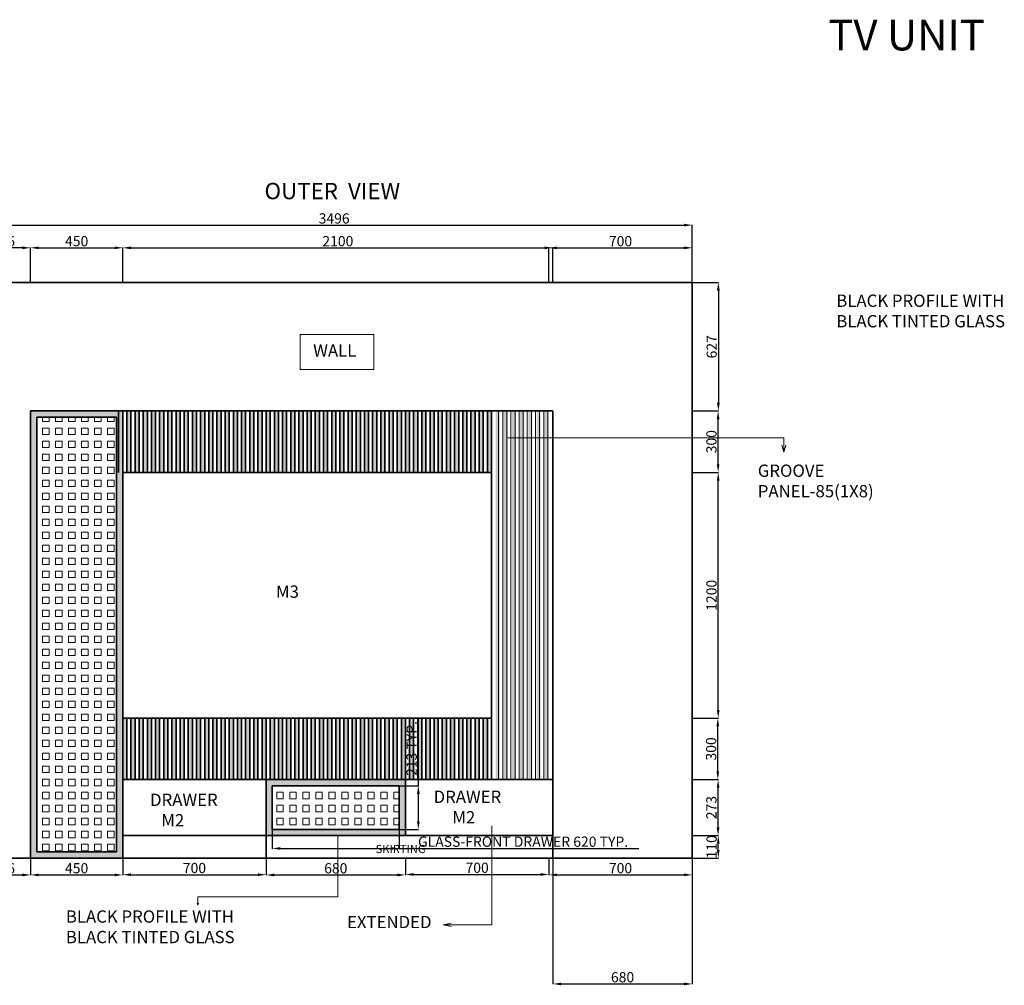
# Model space of a CAD drawing. Units: millimetres. Extents: x 11439 to 24661, y -4767 to -6.
# Tile 2 of 5: x 13922 to 18729, y -4721 to -6. Entities that reach past the tile are written whole.
import ezdxf

# ---------------------------------------------------------------- set-up
doc = ezdxf.new("R2010")
doc.units = ezdxf.units.MM
for name, color, linetype, lineweight in [('A-ANNO-DIMS', 2, 'Continuous', 18), ('A-ANNO-TEXT', 3, 'Continuous', 18), ('A-FURN', 7, 'Continuous', 35), ('A-FURN-PATT', 8, 'Continuous', 13)]:
    doc.layers.add(name, color=color, linetype=linetype, lineweight=lineweight)
doc.styles.get("Standard").update_dxf_attribs({"font": 'arial.ttf'})
doc.dimstyles.new('ISO-25', dxfattribs={"dimtxt": 50, "dimasz": 40, "dimexe": 1.25, "dimexo": 0.625, "dimtad": 1, "dimtxsty": 'Standard', "dimcen": 2.5, "dimadec": 0, "dimazin": 0, "dimtfac": 1, "dimtmove": 0, "dimatfit": 3, "dimfxl": 1, "dimarcsym": 0})

# ---------------------------------------------------------------- blocks, each defined once
blk = doc.blocks.new('*D1')
at = {"layer": 'A-ANNO-DIMS', "color": 0, "lineweight": -2, "transparency": 16777216}
for p, q in [((13708.9, -4100.6), (13708.9, -4183.6)), ((13974.9, -4100.6), (13974.9, -4183.6)), ((13748.9, -4182.3), (13934.9, -4182.3))]:
    blk.add_line(p, q, dxfattribs=at)
at = {"layer": 'A-ANNO-DIMS', "color": 0, "transparency": 16777216}
for points in [[(13748.9, -4175.7), (13748.9, -4189), (13708.9, -4182.3)], [(13934.9, -4175.7), (13934.9, -4189), (13974.9, -4182.3)]]:
    blk.add_solid(points, dxfattribs=at)
at = {"layer": 'Defpoints', "color": 0, "transparency": 16777216}
for p in [(13708.9, -4100), (13974.9, -4100), (13974.9, -4182.3)]:
    blk.add_point(p, dxfattribs=at)
at = {"layer": 'A-ANNO-DIMS', "color": 0, "transparency": 16777216, "insert": (13841.9, -4156.2), "char_height": 50, "attachment_point": 5}
blk.add_mtext('266', dxfattribs=at)
blk = doc.blocks.new('*D2')
at = {"layer": 'A-ANNO-DIMS', "color": 0, "lineweight": -2, "transparency": 16777216}
for p, q in [((13974.9, -4100.6), (13974.9, -4183.6)), ((14424.9, -4100.6), (14424.9, -4183.6)), ((14014.9, -4182.3), (14384.9, -4182.3))]:
    blk.add_line(p, q, dxfattribs=at)
at = {"layer": 'A-ANNO-DIMS', "color": 0, "transparency": 16777216}
for points in [[(14014.9, -4175.7), (14014.9, -4189), (13974.9, -4182.3)], [(14384.9, -4175.7), (14384.9, -4189), (14424.9, -4182.3)]]:
    blk.add_solid(points, dxfattribs=at)
at = {"layer": 'Defpoints', "color": 0, "transparency": 16777216}
for p in [(13974.9, -4100), (14424.9, -4100), (14424.9, -4182.3)]:
    blk.add_point(p, dxfattribs=at)
at = {"layer": 'A-ANNO-DIMS', "color": 0, "transparency": 16777216, "insert": (14199.9, -4156.2), "char_height": 50, "attachment_point": 5}
blk.add_mtext('450', dxfattribs=at)
blk = doc.blocks.new('*D3')
at = {"layer": 'A-ANNO-DIMS', "color": 0, "lineweight": -2, "transparency": 16777216}
for p, q in [((14424.9, -4100.6), (14424.9, -4182.4)), ((15124.9, -4100.6), (15124.9, -4182.4)), ((14464.9, -4181.2), (15084.9, -4181.2))]:
    blk.add_line(p, q, dxfattribs=at)
at = {"layer": 'A-ANNO-DIMS', "color": 0, "transparency": 16777216}
for points in [[(14464.9, -4174.5), (14464.9, -4187.8), (14424.9, -4181.2)], [(15084.9, -4174.5), (15084.9, -4187.8), (15124.9, -4181.2)]]:
    blk.add_solid(points, dxfattribs=at)
at = {"layer": 'Defpoints', "color": 0, "transparency": 16777216}
for p in [(14424.9, -4100), (15124.9, -4100), (15124.9, -4181.2)]:
    blk.add_point(p, dxfattribs=at)
at = {"layer": 'A-ANNO-DIMS', "color": 0, "transparency": 16777216, "insert": (14774.9, -4155), "char_height": 50, "attachment_point": 5}
blk.add_mtext('700', dxfattribs=at)
blk = doc.blocks.new('*D4')
at = {"layer": 'A-ANNO-DIMS', "color": 0, "lineweight": -2, "transparency": 16777216}
for p, q in [((15124.9, -4100.6), (15124.9, -4183.7)), ((15804.9, -4100.6), (15804.9, -4183.7)), ((15164.9, -4182.4), (15764.9, -4182.4))]:
    blk.add_line(p, q, dxfattribs=at)
at = {"layer": 'A-ANNO-DIMS', "color": 0, "transparency": 16777216}
for points in [[(15164.9, -4175.8), (15164.9, -4189.1), (15124.9, -4182.4)], [(15764.9, -4175.8), (15764.9, -4189.1), (15804.9, -4182.4)]]:
    blk.add_solid(points, dxfattribs=at)
at = {"layer": 'Defpoints', "color": 0, "transparency": 16777216}
for p in [(15124.9, -4100), (15804.9, -4100), (15804.9, -4182.4)]:
    blk.add_point(p, dxfattribs=at)
at = {"layer": 'A-ANNO-DIMS', "color": 0, "transparency": 16777216, "insert": (15464.9, -4156.3), "char_height": 50, "attachment_point": 5}
blk.add_mtext('680', dxfattribs=at)
blk = doc.blocks.new('*D5')
at = {"layer": 'A-ANNO-DIMS', "color": 0, "lineweight": -2, "transparency": 16777216}
for p, q in [((15804.9, -4100.6), (15804.9, -4181.3)), ((16504.9, -4100.6), (16504.9, -4181.3)), ((15844.9, -4180), (16464.9, -4180))]:
    blk.add_line(p, q, dxfattribs=at)
at = {"layer": 'A-ANNO-DIMS', "color": 0, "transparency": 16777216}
for points in [[(15844.9, -4173.3), (15844.9, -4186.7), (15804.9, -4180)], [(16464.9, -4173.3), (16464.9, -4186.7), (16504.9, -4180)]]:
    blk.add_solid(points, dxfattribs=at)
at = {"layer": 'Defpoints', "color": 0, "transparency": 16777216}
for p in [(15804.9, -4100), (16504.9, -4100), (16504.9, -4180)]:
    blk.add_point(p, dxfattribs=at)
at = {"layer": 'A-ANNO-DIMS', "color": 0, "transparency": 16777216, "insert": (16154.9, -4153.8), "char_height": 50, "attachment_point": 5}
blk.add_mtext('700', dxfattribs=at)
blk = doc.blocks.new('*D6')
at = {"layer": 'A-ANNO-DIMS', "color": 0, "lineweight": -2, "transparency": 16777216}
for p, q in [((16504.9, -4100.6), (16504.9, -4183.1)), ((17204.9, -4100.6), (17204.9, -4183.1)), ((16544.9, -4181.9), (17164.9, -4181.9))]:
    blk.add_line(p, q, dxfattribs=at)
at = {"layer": 'A-ANNO-DIMS', "color": 0, "transparency": 16777216}
for points in [[(16544.9, -4175.2), (16544.9, -4188.6), (16504.9, -4181.9)], [(17164.9, -4175.2), (17164.9, -4188.6), (17204.9, -4181.9)]]:
    blk.add_solid(points, dxfattribs=at)
at = {"layer": 'Defpoints', "color": 0, "transparency": 16777216}
for p in [(16504.9, -4100), (17204.9, -4100), (17204.9, -4181.9)]:
    blk.add_point(p, dxfattribs=at)
at = {"layer": 'A-ANNO-DIMS', "color": 0, "transparency": 16777216, "insert": (16854.9, -4155.7), "char_height": 50, "attachment_point": 5}
blk.add_mtext('700', dxfattribs=at)
blk = doc.blocks.new('*D7')
at = {"layer": 'A-ANNO-DIMS', "color": 0, "lineweight": -2, "transparency": 16777216}
for p, q in [((17205.5, -3990), (17333.4, -3990)), ((17332.1, -4060), (17332.1, -4030)), ((17205.5, -4100), (17333.4, -4100))]:
    blk.add_line(p, q, dxfattribs=at)
at = {"layer": 'A-ANNO-DIMS', "color": 0, "transparency": 16777216}
for points in [[(17325.5, -4030), (17338.8, -4030), (17332.1, -3990)], [(17325.5, -4060), (17338.8, -4060), (17332.1, -4100)]]:
    blk.add_solid(points, dxfattribs=at)
at = {"layer": 'Defpoints', "color": 0, "transparency": 16777216}
for p in [(17204.9, -3990), (17332.1, -3990), (17204.9, -4100)]:
    blk.add_point(p, dxfattribs=at)
at = {"layer": 'A-ANNO-DIMS', "color": 0, "transparency": 16777216, "insert": (17306, -4045), "char_height": 50, "attachment_point": 5, "rotation": 90}
blk.add_mtext('110', dxfattribs=at)
blk = doc.blocks.new('*D8')
at = {"layer": 'A-ANNO-DIMS', "color": 0, "lineweight": -2, "transparency": 16777216}
for p, q in [((17205.5, -3717), (17332.5, -3717)), ((17331.3, -3950), (17331.3, -3757)), ((17205.5, -3990), (17332.5, -3990))]:
    blk.add_line(p, q, dxfattribs=at)
at = {"layer": 'A-ANNO-DIMS', "color": 0, "transparency": 16777216}
for points in [[(17324.6, -3757), (17338, -3757), (17331.3, -3717)], [(17324.6, -3950), (17338, -3950), (17331.3, -3990)]]:
    blk.add_solid(points, dxfattribs=at)
at = {"layer": 'Defpoints', "color": 0, "transparency": 16777216}
for p in [(17204.9, -3717), (17331.3, -3717), (17204.9, -3990)]:
    blk.add_point(p, dxfattribs=at)
at = {"layer": 'A-ANNO-DIMS', "color": 0, "transparency": 16777216, "insert": (17305.1, -3853.5), "char_height": 50, "attachment_point": 5, "rotation": 90}
blk.add_mtext('273', dxfattribs=at)
blk = doc.blocks.new('*D9')
at = {"layer": 'A-ANNO-DIMS', "color": 0, "lineweight": -2, "transparency": 16777216}
for p, q in [((17205.5, -3417), (17331.1, -3417)), ((17329.9, -3677), (17329.9, -3457)), ((17205.5, -3717), (17331.1, -3717))]:
    blk.add_line(p, q, dxfattribs=at)
at = {"layer": 'A-ANNO-DIMS', "color": 0, "transparency": 16777216}
for points in [[(17323.2, -3457), (17336.5, -3457), (17329.9, -3417)], [(17323.2, -3677), (17336.5, -3677), (17329.9, -3717)]]:
    blk.add_solid(points, dxfattribs=at)
at = {"layer": 'Defpoints', "color": 0, "transparency": 16777216}
for p in [(17204.9, -3417), (17329.9, -3417), (17204.9, -3717)]:
    blk.add_point(p, dxfattribs=at)
at = {"layer": 'A-ANNO-DIMS', "color": 0, "transparency": 16777216, "insert": (17303.7, -3567), "char_height": 50, "attachment_point": 5, "rotation": 90}
blk.add_mtext('300', dxfattribs=at)
blk = doc.blocks.new('*D10')
at = {"layer": 'A-ANNO-DIMS', "color": 0, "lineweight": -2, "transparency": 16777216}
for p, q in [((17205.5, -2217), (17333, -2217)), ((17331.8, -3377), (17331.8, -2257)), ((17205.5, -3417), (17333, -3417))]:
    blk.add_line(p, q, dxfattribs=at)
at = {"layer": 'A-ANNO-DIMS', "color": 0, "transparency": 16777216}
for points in [[(17325.1, -2257), (17338.4, -2257), (17331.8, -2217)], [(17325.1, -3377), (17338.4, -3377), (17331.8, -3417)]]:
    blk.add_solid(points, dxfattribs=at)
at = {"layer": 'Defpoints', "color": 0, "transparency": 16777216}
for p in [(17204.9, -2217), (17331.8, -2217), (17204.9, -3417)]:
    blk.add_point(p, dxfattribs=at)
at = {"layer": 'A-ANNO-DIMS', "color": 0, "transparency": 16777216, "insert": (17305.6, -2817), "char_height": 50, "attachment_point": 5, "rotation": 90}
blk.add_mtext('1200', dxfattribs=at)
blk = doc.blocks.new('*D11')
at = {"layer": 'A-ANNO-DIMS', "color": 0, "lineweight": -2, "transparency": 16777216}
for p, q in [((17209.3, -1917), (17332.6, -1917)), ((17331.4, -2177), (17331.4, -1957)), ((17205.5, -2217), (17332.6, -2217))]:
    blk.add_line(p, q, dxfattribs=at)
at = {"layer": 'A-ANNO-DIMS', "color": 0, "transparency": 16777216}
for points in [[(17324.7, -1957), (17338, -1957), (17331.4, -1917)], [(17324.7, -2177), (17338, -2177), (17331.4, -2217)]]:
    blk.add_solid(points, dxfattribs=at)
at = {"layer": 'Defpoints', "color": 0, "transparency": 16777216}
for p in [(17208.7, -1917), (17331.4, -1917), (17204.9, -2217)]:
    blk.add_point(p, dxfattribs=at)
at = {"layer": 'A-ANNO-DIMS', "color": 0, "transparency": 16777216, "insert": (17305.2, -2067), "char_height": 50, "attachment_point": 5, "rotation": 90}
blk.add_mtext('300', dxfattribs=at)
blk = doc.blocks.new('*D12')
at = {"layer": 'A-ANNO-DIMS', "color": 0, "lineweight": -2, "transparency": 16777216}
for p, q in [((13708.9, -1289.4), (13708.9, -1119.1)), ((13934.9, -1120.3), (13748.9, -1120.3)), ((13974.9, -1289.4), (13974.9, -1119.1))]:
    blk.add_line(p, q, dxfattribs=at)
at = {"layer": 'A-ANNO-DIMS', "color": 0, "transparency": 16777216}
for points in [[(13748.9, -1113.7), (13748.9, -1127), (13708.9, -1120.3)], [(13934.9, -1113.7), (13934.9, -1127), (13974.9, -1120.3)]]:
    blk.add_solid(points, dxfattribs=at)
at = {"layer": 'Defpoints', "color": 0, "transparency": 16777216}
for p in [(13708.9, -1120.3), (13708.9, -1290), (13974.9, -1290)]:
    blk.add_point(p, dxfattribs=at)
at = {"layer": 'A-ANNO-DIMS', "color": 0, "transparency": 16777216, "insert": (13841.9, -1094.2), "char_height": 50, "attachment_point": 5}
blk.add_mtext('266', dxfattribs=at)
blk = doc.blocks.new('*D13')
at = {"layer": 'A-ANNO-DIMS', "color": 0, "lineweight": -2, "transparency": 16777216}
for p, q in [((13974.9, -1289.4), (13974.9, -1119.1)), ((14014.9, -1120.3), (14384.9, -1120.3)), ((14424.9, -1289.4), (14424.9, -1119.1))]:
    blk.add_line(p, q, dxfattribs=at)
at = {"layer": 'A-ANNO-DIMS', "color": 0, "transparency": 16777216}
for points in [[(14014.9, -1113.7), (14014.9, -1127), (13974.9, -1120.3)], [(14384.9, -1113.7), (14384.9, -1127), (14424.9, -1120.3)]]:
    blk.add_solid(points, dxfattribs=at)
at = {"layer": 'Defpoints', "color": 0, "transparency": 16777216}
for p in [(14424.9, -1120.3), (13974.9, -1290), (14424.9, -1290)]:
    blk.add_point(p, dxfattribs=at)
at = {"layer": 'A-ANNO-DIMS', "color": 0, "transparency": 16777216, "insert": (14199.9, -1094.2), "char_height": 50, "attachment_point": 5}
blk.add_mtext('450', dxfattribs=at)
blk = doc.blocks.new('*D14')
at = {"layer": 'A-ANNO-DIMS', "color": 0, "lineweight": -2, "transparency": 16777216}
for p, q in [((14424.9, -1289.4), (14424.9, -1119.2)), ((14464.9, -1120.4), (16484.9, -1120.4)), ((16524.9, -1289.4), (16524.9, -1119.2))]:
    blk.add_line(p, q, dxfattribs=at)
at = {"layer": 'A-ANNO-DIMS', "color": 0, "transparency": 16777216}
for points in [[(14464.9, -1113.8), (14464.9, -1127.1), (14424.9, -1120.4)], [(16484.9, -1113.8), (16484.9, -1127.1), (16524.9, -1120.4)]]:
    blk.add_solid(points, dxfattribs=at)
at = {"layer": 'Defpoints', "color": 0, "transparency": 16777216}
for p in [(16524.9, -1120.4), (14424.9, -1290), (16524.9, -1290)]:
    blk.add_point(p, dxfattribs=at)
at = {"layer": 'A-ANNO-DIMS', "color": 0, "transparency": 16777216, "insert": (15474.9, -1094.3), "char_height": 50, "attachment_point": 5}
blk.add_mtext('2100', dxfattribs=at)
blk = doc.blocks.new('*D15')
at = {"layer": 'A-ANNO-DIMS', "color": 0, "lineweight": -2, "transparency": 16777216}
for p, q in [((16504.9, -1289.4), (16504.9, -1119.2)), ((16544.9, -1120.4), (17164.9, -1120.4)), ((17204.9, -1289.4), (17204.9, -1119.2))]:
    blk.add_line(p, q, dxfattribs=at)
at = {"layer": 'A-ANNO-DIMS', "color": 0, "transparency": 16777216}
for points in [[(16544.9, -1113.8), (16544.9, -1127.1), (16504.9, -1120.4)], [(17164.9, -1113.8), (17164.9, -1127.1), (17204.9, -1120.4)]]:
    blk.add_solid(points, dxfattribs=at)
at = {"layer": 'Defpoints', "color": 0, "transparency": 16777216}
for p in [(17204.9, -1120.4), (16504.9, -1290), (17204.9, -1290)]:
    blk.add_point(p, dxfattribs=at)
at = {"layer": 'A-ANNO-DIMS', "color": 0, "transparency": 16777216, "insert": (16854.9, -1094.3), "char_height": 50, "attachment_point": 5}
blk.add_mtext('700', dxfattribs=at)
blk = doc.blocks.new('*D16')
at = {"layer": 'A-ANNO-DIMS', "color": 0, "lineweight": -2, "transparency": 16777216}
for p, q in [((17205.5, -1290), (17333.9, -1290)), ((17332.6, -1330), (17332.6, -1877)), ((17209.3, -1917), (17333.9, -1917))]:
    blk.add_line(p, q, dxfattribs=at)
at = {"layer": 'A-ANNO-DIMS', "color": 0, "transparency": 16777216}
for points in [[(17325.9, -1330), (17339.3, -1330), (17332.6, -1290)], [(17325.9, -1877), (17339.3, -1877), (17332.6, -1917)]]:
    blk.add_solid(points, dxfattribs=at)
at = {"layer": 'Defpoints', "color": 0, "transparency": 16777216}
for p in [(17204.9, -1290), (17208.7, -1917), (17332.6, -1917)]:
    blk.add_point(p, dxfattribs=at)
at = {"layer": 'A-ANNO-DIMS', "color": 0, "transparency": 16777216, "insert": (17306.5, -1603.5), "char_height": 50, "attachment_point": 5, "rotation": 90}
blk.add_mtext('627', dxfattribs=at)
blk = doc.blocks.new('DRAWER-GLASS-FRONT')
for p, q in [((0, 213), (620, 213)), ((0, 0), (0, 213)), ((620, 0), (620, 213)), ((0, 0), (620, 0))]:
    blk.add_line(p, q)
blk = doc.blocks.new('*D49')
at = {"layer": 'A-ANNO-DIMS', "color": 0, "lineweight": -2, "transparency": 16777216}
for p, q in [((15154.9, -3960.6), (15154.9, -4054.2)), ((15774.9, -3960.6), (15774.9, -4054.2)), ((15194.9, -4053), (15734.9, -4053)), ((15774.9, -4053), (16943.6, -4053))]:
    blk.add_line(p, q, dxfattribs=at)
at = {"layer": 'A-ANNO-DIMS', "color": 0, "transparency": 16777216}
for points in [[(15194.9, -4046.3), (15194.9, -4059.7), (15154.9, -4053)], [(15734.9, -4046.3), (15734.9, -4059.7), (15774.9, -4053)]]:
    blk.add_solid(points, dxfattribs=at)
at = {"layer": 'Defpoints', "color": 0, "transparency": 16777216}
for p in [(15154.9, -3960), (15774.9, -3960), (15774.9, -4053)]:
    blk.add_point(p, dxfattribs=at)
at = {"layer": 'A-ANNO-DIMS', "color": 0, "transparency": 16777216, "insert": (16379.3, -4026.5), "char_height": 50, "attachment_point": 5}
blk.add_mtext('GLASS-FRONT DRAWER 620 TYP.', dxfattribs=at)
blk = doc.blocks.new('*D50')
at = {"layer": 'A-ANNO-DIMS', "color": 0, "lineweight": -2, "transparency": 16777216}
for p, q in [((15867.9, -3747), (15867.9, -3422.7)), ((15775.5, -3747), (15869.2, -3747)), ((15867.9, -3920), (15867.9, -3787)), ((15775.5, -3960), (15869.2, -3960))]:
    blk.add_line(p, q, dxfattribs=at)
at = {"layer": 'A-ANNO-DIMS', "color": 0, "transparency": 16777216}
for points in [[(15861.2, -3787), (15874.6, -3787), (15867.9, -3747)], [(15861.2, -3920), (15874.6, -3920), (15867.9, -3960)]]:
    blk.add_solid(points, dxfattribs=at)
at = {"layer": 'Defpoints', "color": 0, "transparency": 16777216}
for p in [(15774.9, -3747), (15867.9, -3747), (15774.9, -3960)]:
    blk.add_point(p, dxfattribs=at)
at = {"layer": 'A-ANNO-DIMS', "color": 0, "transparency": 16777216, "insert": (15841.7, -3564.8), "char_height": 50, "attachment_point": 5, "rotation": 90}
blk.add_mtext('213 TYP.', dxfattribs=at)
blk = doc.blocks.new('*D57')
at = {"layer": 'A-ANNO-DIMS', "color": 0, "lineweight": -2, "transparency": 16777216}
for p, q in [((16524.9, -4100.6), (16524.9, -4715.8)), ((17204.9, -4100.6), (17204.9, -4715.8)), ((16564.9, -4714.6), (17164.9, -4714.6))]:
    blk.add_line(p, q, dxfattribs=at)
at = {"layer": 'A-ANNO-DIMS', "color": 0, "transparency": 16777216}
for points in [[(16564.9, -4707.9), (16564.9, -4721.2), (16524.9, -4714.6)], [(17164.9, -4707.9), (17164.9, -4721.2), (17204.9, -4714.6)]]:
    blk.add_solid(points, dxfattribs=at)
at = {"layer": 'Defpoints', "color": 0, "transparency": 16777216}
for p in [(16524.9, -4100), (17204.9, -4100), (17204.9, -4714.6)]:
    blk.add_point(p, dxfattribs=at)
at = {"layer": 'A-ANNO-DIMS', "color": 0, "transparency": 16777216, "insert": (16864.9, -4688.4), "char_height": 50, "attachment_point": 5}
blk.add_mtext('680', dxfattribs=at)
blk = doc.blocks.new('*D58')
at = {"layer": 'A-ANNO-DIMS', "color": 0, "lineweight": -2, "transparency": 16777216}
for p, q in [((13708.9, -1289.4), (13708.9, -1008.2)), ((17204.9, -1289.4), (17204.9, -1008.2)), ((13748.9, -1009.5), (17164.9, -1009.5))]:
    blk.add_line(p, q, dxfattribs=at)
at = {"layer": 'A-ANNO-DIMS', "color": 0, "transparency": 16777216}
for points in [[(13748.9, -1002.8), (13748.9, -1016.2), (13708.9, -1009.5)], [(17164.9, -1002.8), (17164.9, -1016.2), (17204.9, -1009.5)]]:
    blk.add_solid(points, dxfattribs=at)
at = {"layer": 'Defpoints', "color": 0, "transparency": 16777216}
for p in [(17204.9, -1009.5), (13708.9, -1290), (17204.9, -1290)]:
    blk.add_point(p, dxfattribs=at)
at = {"layer": 'A-ANNO-DIMS', "color": 0, "transparency": 16777216, "insert": (15456.9, -983.3), "char_height": 50, "attachment_point": 5}
blk.add_mtext('3496', dxfattribs=at)

msp = doc.modelspace()

# ---------------------------------------------------------------- hatches: boundary and pattern name
at = {"layer": 'A-FURN-PATT'}
h = msp.add_hatch(color=256, dxfattribs=at)
h.dxf.hatch_style = 1
h.paths.add_polyline_path([(13974.915, -4099.995), (14424.915, -4099.995), (14424.915, -1916.995), (13974.915, -1916.995)])
h.paths.add_polyline_path([(14004.915, -1946.995), (14394.915, -1946.995), (14394.915, -4069.995), (14004.915, -4069.995)], flags=16)
h = msp.add_hatch(color=256, dxfattribs=at)
h.dxf.hatch_style = 1
h.paths.add_polyline_path([(14464.915, -1916.995), (14444.915, -1916.995), (14444.915, -2216.995), (14464.915, -2216.995)])
h = msp.add_hatch(color=256, dxfattribs=at)
h.dxf.hatch_style = 1
h.paths.add_polyline_path([(14504.915, -1916.995), (14484.915, -1916.995), (14484.915, -2216.995), (14504.915, -2216.995)])
h.paths.add_polyline_path([(14544.915, -1916.995), (14524.915, -1916.995), (14524.915, -2216.995), (14544.915, -2216.995)])
h.paths.add_polyline_path([(14584.915, -1916.995), (14564.915, -1916.995), (14564.915, -2216.995), (14584.915, -2216.995)])
h.paths.add_polyline_path([(14624.915, -1916.995), (14604.915, -1916.995), (14604.915, -2216.995), (14624.915, -2216.995)])
h.paths.add_polyline_path([(14664.915, -1916.995), (14644.915, -1916.995), (14644.915, -2216.995), (14664.915, -2216.995)])
h.paths.add_polyline_path([(14704.915, -1916.995), (14684.915, -1916.995), (14684.915, -2216.995), (14704.915, -2216.995)])
h.paths.add_polyline_path([(14744.915, -1916.995), (14724.915, -1916.995), (14724.915, -2216.995), (14744.915, -2216.995)])
h.paths.add_polyline_path([(14784.915, -1916.995), (14764.915, -1916.995), (14764.915, -2216.995), (14784.915, -2216.995)])
h.paths.add_polyline_path([(14824.915, -1916.995), (14804.915, -1916.995), (14804.915, -2216.995), (14824.915, -2216.995)])
h.paths.add_polyline_path([(14864.915, -1916.995), (14844.915, -1916.995), (14844.915, -2216.995), (14864.915, -2216.995)])
h.paths.add_polyline_path([(14904.915, -1916.995), (14884.915, -1916.995), (14884.915, -2216.995), (14904.915, -2216.995)])
h.paths.add_polyline_path([(14944.915, -1916.995), (14924.915, -1916.995), (14924.915, -2216.995), (14944.915, -2216.995)])
h.paths.add_polyline_path([(14984.915, -1916.995), (14964.915, -1916.995), (14964.915, -2216.995), (14984.915, -2216.995)])
h.paths.add_polyline_path([(15024.915, -1916.995), (15004.915, -1916.995), (15004.915, -2216.995), (15024.915, -2216.995)])
h.paths.add_polyline_path([(15064.915, -1916.995), (15044.915, -1916.995), (15044.915, -2216.995), (15064.915, -2216.995)])
h.paths.add_polyline_path([(15104.915, -1916.995), (15084.915, -1916.995), (15084.915, -2216.995), (15104.915, -2216.995)])
h.paths.add_polyline_path([(15144.915, -1916.995), (15124.915, -1916.995), (15124.915, -2216.995), (15144.915, -2216.995)])
h.paths.add_polyline_path([(15184.915, -1916.995), (15164.915, -1916.995), (15164.915, -2216.995), (15184.915, -2216.995)])
h.paths.add_polyline_path([(15224.915, -1916.995), (15204.915, -1916.995), (15204.915, -2216.995), (15224.915, -2216.995)])
h.paths.add_polyline_path([(15264.915, -1916.995), (15244.915, -1916.995), (15244.915, -2216.995), (15264.915, -2216.995)])
h.paths.add_polyline_path([(15304.915, -1916.995), (15284.915, -1916.995), (15284.915, -2216.995), (15304.915, -2216.995)])
h.paths.add_polyline_path([(15344.915, -1916.995), (15324.915, -1916.995), (15324.915, -2216.995), (15344.915, -2216.995)])
h.paths.add_polyline_path([(15384.915, -1916.995), (15364.915, -1916.995), (15364.915, -2216.995), (15384.915, -2216.995)])
h.paths.add_polyline_path([(15424.915, -1916.995), (15404.915, -1916.995), (15404.915, -2216.995), (15424.915, -2216.995)])
h.paths.add_polyline_path([(15464.915, -1916.995), (15444.915, -1916.995), (15444.915, -2216.995), (15464.915, -2216.995)])
h.paths.add_polyline_path([(15504.915, -1916.995), (15484.915, -1916.995), (15484.915, -2216.995), (15504.915, -2216.995)])
h.paths.add_polyline_path([(15544.915, -1916.995), (15524.915, -1916.995), (15524.915, -2216.995), (15544.915, -2216.995)])
h.paths.add_polyline_path([(15584.915, -1916.995), (15564.915, -1916.995), (15564.915, -2216.995), (15584.915, -2216.995)])
h.paths.add_polyline_path([(15624.915, -1916.995), (15604.915, -1916.995), (15604.915, -2216.995), (15624.915, -2216.995)])
h.paths.add_polyline_path([(15664.915, -1916.995), (15644.915, -1916.995), (15644.915, -2216.995), (15664.915, -2216.995)])
h.paths.add_polyline_path([(15704.915, -1916.995), (15684.915, -1916.995), (15684.915, -2216.995), (15704.915, -2216.995)])
h.paths.add_polyline_path([(15744.915, -1916.995), (15724.915, -1916.995), (15724.915, -2216.995), (15744.915, -2216.995)])
h.paths.add_polyline_path([(15784.915, -1916.995), (15764.915, -1916.995), (15764.915, -2216.995), (15784.915, -2216.995)])
h.paths.add_polyline_path([(15824.915, -1916.995), (15804.915, -1916.995), (15804.915, -2216.995), (15824.915, -2216.995)])
h.paths.add_polyline_path([(15864.915, -1916.995), (15844.915, -1916.995), (15844.915, -2216.995), (15864.915, -2216.995)])
h.paths.add_polyline_path([(15904.915, -1916.995), (15884.915, -1916.995), (15884.915, -2216.995), (15904.915, -2216.995)])
h.paths.add_polyline_path([(15944.915, -1916.995), (15924.915, -1916.995), (15924.915, -2216.995), (15944.915, -2216.995)])
h.paths.add_polyline_path([(15984.915, -1916.995), (15964.915, -1916.995), (15964.915, -2216.995), (15984.915, -2216.995)])
h.paths.add_polyline_path([(16024.915, -1916.995), (16004.915, -1916.995), (16004.915, -2216.995), (16024.915, -2216.995)])
h.paths.add_polyline_path([(16064.915, -1916.995), (16044.915, -1916.995), (16044.915, -2216.995), (16064.915, -2216.995)])
h.paths.add_polyline_path([(16104.915, -1916.995), (16084.915, -1916.995), (16084.915, -2216.995), (16104.915, -2216.995)])
h.paths.add_polyline_path([(16144.915, -1916.995), (16124.915, -1916.995), (16124.915, -2216.995), (16144.915, -2216.995)])
h.paths.add_polyline_path([(16184.915, -1916.995), (16164.915, -1916.995), (16164.915, -2216.995), (16184.915, -2216.995)])
h.paths.add_polyline_path([(16224.915, -1916.995), (16204.915, -1916.995), (16204.915, -2216.995), (16224.915, -2216.995)])
h = msp.add_hatch(color=256, dxfattribs=at)
h.dxf.hatch_style = 1
h.paths.add_polyline_path([(16264.915, -1916.995), (16244.915, -1916.995), (16244.915, -3716.995), (16264.915, -3716.995)])
h.paths.add_polyline_path([(16304.915, -1916.995), (16284.915, -1916.995), (16284.915, -3716.995), (16304.915, -3716.995)])
h.paths.add_polyline_path([(16344.915, -1916.995), (16324.915, -1916.995), (16324.915, -2047.953), (16344.915, -2047.953)])
h.paths.add_polyline_path([(16344.915, -2047.953), (16324.915, -2047.953), (16324.915, -3716.995), (16344.915, -3716.995)])
h.paths.add_polyline_path([(16384.915, -2047.953), (16364.915, -2047.953), (16364.915, -3716.995), (16384.915, -3716.995)])
h.paths.add_polyline_path([(16384.915, -1916.995), (16364.915, -1916.995), (16364.915, -2047.953), (16384.915, -2047.953)])
h.paths.add_polyline_path([(16424.915, -1916.995), (16404.915, -1916.995), (16404.915, -2047.953), (16424.915, -2047.953)])
h.paths.add_polyline_path([(16424.915, -2047.953), (16404.915, -2047.953), (16404.915, -3716.995), (16424.915, -3716.995)])
h.paths.add_polyline_path([(16464.915, -2047.953), (16444.915, -2047.953), (16444.915, -3716.995), (16464.915, -3716.995)])
h.paths.add_polyline_path([(16464.915, -1916.995), (16444.915, -1916.995), (16444.915, -2047.953), (16464.915, -2047.953)])
h.paths.add_polyline_path([(16504.915, -2047.953), (16484.915, -2047.953), (16484.915, -3716.995), (16504.915, -3716.995)])
h.paths.add_polyline_path([(16504.915, -1916.995), (16484.915, -1916.995), (16484.915, -2047.953), (16504.915, -2047.953)])
h = msp.add_hatch(dxfattribs=at)
h.set_pattern_fill('ANSI31', color=256, scale=6.29921, angle=45, style=0)
h.paths.add_polyline_path([(16244.915, -3716.995), (16504.915, -3716.995), (16504.915, -1916.995), (16244.915, -1916.995)])
h = msp.add_hatch(dxfattribs=at)
h.set_pattern_fill('SQUARE', color=256, scale=10)
h.paths.add_polyline_path([(14394.915, -1946.995), (14004.915, -1946.995), (14004.915, -4069.995), (14394.915, -4069.995)])
h = msp.add_hatch(color=256, dxfattribs=at)
h.dxf.hatch_style = 1
h.paths.add_polyline_path([(14444.915, -3416.995), (14424.915, -3416.995), (14424.915, -3716.995), (14444.915, -3716.995)])
h.paths.add_polyline_path([(14484.915, -3416.995), (14464.915, -3416.995), (14464.915, -3716.995), (14484.915, -3716.995)])
h.paths.add_polyline_path([(14524.915, -3416.995), (14504.915, -3416.995), (14504.915, -3716.995), (14524.915, -3716.995)])
h.paths.add_polyline_path([(14564.915, -3416.995), (14544.915, -3416.995), (14544.915, -3716.995), (14564.915, -3716.995)])
h.paths.add_polyline_path([(14604.915, -3416.995), (14584.915, -3416.995), (14584.915, -3716.995), (14604.915, -3716.995)])
h.paths.add_polyline_path([(14644.915, -3416.995), (14624.915, -3416.995), (14624.915, -3716.995), (14644.915, -3716.995)])
h.paths.add_polyline_path([(14684.915, -3416.995), (14664.915, -3416.995), (14664.915, -3716.995), (14684.915, -3716.995)])
h.paths.add_polyline_path([(14724.915, -3416.995), (14704.915, -3416.995), (14704.915, -3716.995), (14724.915, -3716.995)])
h.paths.add_polyline_path([(14764.915, -3416.995), (14744.915, -3416.995), (14744.915, -3716.995), (14764.915, -3716.995)])
h.paths.add_polyline_path([(14804.915, -3416.995), (14784.915, -3416.995), (14784.915, -3716.995), (14804.915, -3716.995)])
h.paths.add_polyline_path([(14844.915, -3416.995), (14824.915, -3416.995), (14824.915, -3716.995), (14844.915, -3716.995)])
h.paths.add_polyline_path([(14884.915, -3416.995), (14864.915, -3416.995), (14864.915, -3716.995), (14884.915, -3716.995)])
h.paths.add_polyline_path([(14924.915, -3416.995), (14904.915, -3416.995), (14904.915, -3716.995), (14924.915, -3716.995)])
h.paths.add_polyline_path([(14964.915, -3416.995), (14944.915, -3416.995), (14944.915, -3716.995), (14964.915, -3716.995)])
h.paths.add_polyline_path([(15004.915, -3416.995), (14984.915, -3416.995), (14984.915, -3716.995), (15004.915, -3716.995)])
h.paths.add_polyline_path([(15044.915, -3416.995), (15024.915, -3416.995), (15024.915, -3716.995), (15044.915, -3716.995)])
h.paths.add_polyline_path([(15084.915, -3416.995), (15064.915, -3416.995), (15064.915, -3716.995), (15084.915, -3716.995)])
h.paths.add_polyline_path([(15124.915, -3416.995), (15104.915, -3416.995), (15104.915, -3716.995), (15124.915, -3716.995)])
h.paths.add_polyline_path([(15164.915, -3416.995), (15144.915, -3416.995), (15144.915, -3716.995), (15164.915, -3716.995)])
h.paths.add_polyline_path([(15204.915, -3416.995), (15184.915, -3416.995), (15184.915, -3716.995), (15204.915, -3716.995)])
h.paths.add_polyline_path([(15244.915, -3416.995), (15224.915, -3416.995), (15224.915, -3716.995), (15244.915, -3716.995)])
h.paths.add_polyline_path([(15284.915, -3416.995), (15264.915, -3416.995), (15264.915, -3716.995), (15284.915, -3716.995)])
h.paths.add_polyline_path([(15324.915, -3416.995), (15304.915, -3416.995), (15304.915, -3716.995), (15324.915, -3716.995)])
h.paths.add_polyline_path([(15364.915, -3416.995), (15344.915, -3416.995), (15344.915, -3716.995), (15364.915, -3716.995)])
h.paths.add_polyline_path([(15404.915, -3416.995), (15384.915, -3416.995), (15384.915, -3716.995), (15404.915, -3716.995)])
h.paths.add_polyline_path([(15444.915, -3416.995), (15424.915, -3416.995), (15424.915, -3716.995), (15444.915, -3716.995)])
h.paths.add_polyline_path([(15484.915, -3416.995), (15464.915, -3416.995), (15464.915, -3716.995), (15484.915, -3716.995)])
h.paths.add_polyline_path([(15524.915, -3416.995), (15504.915, -3416.995), (15504.915, -3716.995), (15524.915, -3716.995)])
h.paths.add_polyline_path([(15564.915, -3416.995), (15544.915, -3416.995), (15544.915, -3716.995), (15564.915, -3716.995)])
h.paths.add_polyline_path([(15604.915, -3416.995), (15584.915, -3416.995), (15584.915, -3716.995), (15604.915, -3716.995)])
h.paths.add_polyline_path([(15644.915, -3416.995), (15624.915, -3416.995), (15624.915, -3716.995), (15644.915, -3716.995)])
h.paths.add_polyline_path([(15684.915, -3416.995), (15664.915, -3416.995), (15664.915, -3716.995), (15684.915, -3716.995)])
h.paths.add_polyline_path([(15724.915, -3416.995), (15704.915, -3416.995), (15704.915, -3716.995), (15724.915, -3716.995)])
h.paths.add_polyline_path([(15764.915, -3416.995), (15744.915, -3416.995), (15744.915, -3716.995), (15764.915, -3716.995)])
h.paths.add_polyline_path([(15804.915, -3416.995), (15784.915, -3416.995), (15784.915, -3716.995), (15804.915, -3716.995)])
h.paths.add_polyline_path([(15844.915, -3416.995), (15824.915, -3416.995), (15824.915, -3716.995), (15844.915, -3716.995)])
h.paths.add_polyline_path([(15884.915, -3416.995), (15864.915, -3416.995), (15864.915, -3716.995), (15884.915, -3716.995)])
h.paths.add_polyline_path([(15924.915, -3416.995), (15904.915, -3416.995), (15904.915, -3716.995), (15924.915, -3716.995)])
h.paths.add_polyline_path([(15964.915, -3416.995), (15944.915, -3416.995), (15944.915, -3716.995), (15964.915, -3716.995)])
h.paths.add_polyline_path([(16004.915, -3416.995), (15984.915, -3416.995), (15984.915, -3716.995), (16004.915, -3716.995)])
h.paths.add_polyline_path([(16044.915, -3416.995), (16024.915, -3416.995), (16024.915, -3716.995), (16044.915, -3716.995)])
h.paths.add_polyline_path([(16084.915, -3416.995), (16064.915, -3416.995), (16064.915, -3716.995), (16084.915, -3716.995)])
h.paths.add_polyline_path([(16124.915, -3416.995), (16104.915, -3416.995), (16104.915, -3716.995), (16124.915, -3716.995)])
h.paths.add_polyline_path([(16164.915, -3416.995), (16144.915, -3416.995), (16144.915, -3716.995), (16164.915, -3716.995)])
h.paths.add_polyline_path([(16204.915, -3416.995), (16184.915, -3416.995), (16184.915, -3716.995), (16204.915, -3716.995)])
h = msp.add_hatch(color=256, dxfattribs=at)
h.dxf.hatch_style = 1
h.paths.add_polyline_path([(15804.915, -3989.995), (15804.915, -3716.995), (15124.915, -3716.995), (15124.915, -3989.995)])
h.paths.add_polyline_path([(15154.915, -3959.995), (15154.915, -3746.995), (15774.915, -3746.995), (15774.915, -3959.995)], flags=16)
h = msp.add_hatch(dxfattribs=at)
h.set_pattern_fill('SQUARE', color=256, scale=10)
h.paths.add_polyline_path([(15774.915, -3746.995), (15154.915, -3746.995), (15154.915, -3959.995), (15774.915, -3959.995)])

# ---------------------------------------------------------------- linework, layer by layer
at = {"layer": 'A-ANNO-TEXT'}
for p, q in [((16304.915, -2047.953), (16304.915, -2047.953)), ((16304.915, -2047.953), (17651.688, -2047.953)), ((17651.688, -2047.953), (17651.688, -2118.822)), ((17651.688, -2118.822), (17642.208, -2084.333)), ((17651.688, -2118.822), (17661.416, -2083.419)), ((16226.224, -3942.125), (16226.224, -4425.71)), ((15474.915, -3989.995), (15474.915, -4289.242)), ((14792.131, -4329.892), (14788.722, -4319.304)), ((15474.915, -4289.242), (14792.131, -4289.242)), ((14792.131, -4289.242), (14792.131, -4329.892)), ((14792.131, -4329.892), (14795.396, -4319.622)), ((15989.686, -4425.71), (16028.206, -4417.919)), ((16226.224, -4425.71), (15989.686, -4425.71)), ((15989.686, -4425.71), (16029.321, -4434.071))]:
    msp.add_line(p, q, dxfattribs=at)
msp.add_lwpolyline([(15291.366, -1544.351), (15650.752, -1544.351), (15650.752, -1713.672), (15291.366, -1713.672)], close=True, dxfattribs=at)
at = {"layer": 'A-FURN'}
for p, q in [((13708.915, -1289.995), (17204.915, -1289.995)), ((17204.915, -4099.995), (17204.915, -1289.995)), ((13974.915, -4099.995), (13974.915, -1916.995)), ((13974.915, -1916.995), (16524.915, -1916.995)), ((14404.915, -2216.995), (14404.915, -1916.995)), ((14424.915, -4099.995), (14424.915, -1916.995)), ((14424.915, -2216.995), (14424.915, -1916.995)), ((14444.915, -2216.995), (14444.915, -1916.995)), ((14464.915, -2216.995), (14464.915, -1916.995)), ((14484.915, -2216.995), (14484.915, -1916.995)), ((14504.915, -2216.995), (14504.915, -1916.995)), ((14524.915, -2216.995), (14524.915, -1916.995)), ((14544.915, -2216.995), (14544.915, -1916.995)), ((14564.915, -2216.995), (14564.915, -1916.995)), ((14584.915, -2216.995), (14584.915, -1916.995)), ((14604.915, -2216.995), (14604.915, -1916.995)), ((14624.915, -2216.995), (14624.915, -1916.995)), ((14644.915, -2216.995), (14644.915, -1916.995)), ((14664.915, -2216.995), (14664.915, -1916.995)), ((14684.915, -2216.995), (14684.915, -1916.995)), ((14704.915, -2216.995), (14704.915, -1916.995)), ((14724.915, -2216.995), (14724.915, -1916.995)), ((14744.915, -2216.995), (14744.915, -1916.995)), ((14764.915, -2216.995), (14764.915, -1916.995)), ((14784.915, -2216.995), (14784.915, -1916.995)), ((14804.915, -2216.995), (14804.915, -1916.995)), ((14824.915, -2216.995), (14824.915, -1916.995)), ((14844.915, -2216.995), (14844.915, -1916.995)), ((14864.915, -2216.995), (14864.915, -1916.995)), ((14884.915, -2216.995), (14884.915, -1916.995)), ((14904.915, -2216.995), (14904.915, -1916.995)), ((14924.915, -2216.995), (14924.915, -1916.995)), ((14944.915, -2216.995), (14944.915, -1916.995)), ((14964.915, -2216.995), (14964.915, -1916.995)), ((14984.915, -2216.995), (14984.915, -1916.995)), ((15004.915, -2216.995), (15004.915, -1916.995)), ((15024.915, -2216.995), (15024.915, -1916.995)), ((15044.915, -2216.995), (15044.915, -1916.995)), ((15064.915, -2216.995), (15064.915, -1916.995)), ((15084.915, -2216.995), (15084.915, -1916.995)), ((15104.915, -2216.995), (15104.915, -1916.995)), ((15124.915, -2216.995), (15124.915, -1916.995)), ((15144.915, -2216.995), (15144.915, -1916.995)), ((15164.915, -2216.995), (15164.915, -1916.995)), ((15184.915, -2216.995), (15184.915, -1916.995)), ((15204.915, -2216.995), (15204.915, -1916.995)), ((15224.915, -2216.995), (15224.915, -1916.995)), ((15244.915, -2216.995), (15244.915, -1916.995)), ((15264.915, -2216.995), (15264.915, -1916.995)), ((15284.915, -2216.995), (15284.915, -1916.995)), ((15304.915, -2216.995), (15304.915, -1916.995)), ((15324.915, -2216.995), (15324.915, -1916.995)), ((15344.915, -2216.995), (15344.915, -1916.995)), ((15364.915, -2216.995), (15364.915, -1916.995)), ((15384.915, -2216.995), (15384.915, -1916.995)), ((15404.915, -2216.995), (15404.915, -1916.995)), ((15424.915, -2216.995), (15424.915, -1916.995)), ((15444.915, -2216.995), (15444.915, -1916.995)), ((15464.915, -2216.995), (15464.915, -1916.995)), ((15484.915, -2216.995), (15484.915, -1916.995)), ((15504.915, -2216.995), (15504.915, -1916.995)), ((15524.915, -2216.995), (15524.915, -1916.995)), ((15544.915, -2216.995), (15544.915, -1916.995)), ((15564.915, -2216.995), (15564.915, -1916.995)), ((15584.915, -2216.995), (15584.915, -1916.995)), ((15604.915, -2216.995), (15604.915, -1916.995)), ((15624.915, -2216.995), (15624.915, -1916.995)), ((15644.915, -2216.995), (15644.915, -1916.995)), ((15664.915, -2216.995), (15664.915, -1916.995)), ((15684.915, -2216.995), (15684.915, -1916.995)), ((15704.915, -2216.995), (15704.915, -1916.995)), ((15724.915, -2216.995), (15724.915, -1916.995)), ((15744.915, -2216.995), (15744.915, -1916.995)), ((15764.915, -2216.995), (15764.915, -1916.995)), ((15784.915, -2216.995), (15784.915, -1916.995)), ((15804.915, -2216.995), (15804.915, -1916.995)), ((15824.915, -2216.995), (15824.915, -1916.995)), ((15844.915, -2216.995), (15844.915, -1916.995)), ((15864.915, -2216.995), (15864.915, -1916.995)), ((15884.915, -2216.995), (15884.915, -1916.995)), ((15904.915, -2216.995), (15904.915, -1916.995)), ((15924.915, -2216.995), (15924.915, -1916.995)), ((15944.915, -2216.995), (15944.915, -1916.995)), ((15964.915, -2216.995), (15964.915, -1916.995)), ((15984.915, -2216.995), (15984.915, -1916.995)), ((16004.915, -2216.995), (16004.915, -1916.995)), ((16024.915, -2216.995), (16024.915, -1916.995)), ((16044.915, -2216.995), (16044.915, -1916.995)), ((16064.915, -2216.995), (16064.915, -1916.995)), ((16084.915, -2216.995), (16084.915, -1916.995)), ((16104.915, -2216.995), (16104.915, -1916.995)), ((16124.915, -2216.995), (16124.915, -1916.995)), ((16144.915, -2216.995), (16144.915, -1916.995)), ((16164.915, -2216.995), (16164.915, -1916.995)), ((16184.915, -2216.995), (16184.915, -1916.995)), ((16204.915, -2216.995), (16204.915, -1916.995)), ((16224.915, -2216.995), (16224.915, -1916.995)), ((16524.915, -4099.995), (16524.915, -1916.995)), ((14004.915, -4069.995), (14004.915, -1946.995)), ((14004.915, -1946.995), (14394.915, -1946.995)), ((14394.915, -4069.995), (14394.915, -1946.995)), ((14424.915, -2216.995), (16224.915, -2216.995)), ((16224.915, -3416.995), (16224.915, -2216.995)), ((14424.915, -3416.995), (16224.915, -3416.995)), ((14444.915, -3716.995), (14444.915, -3416.995)), ((14464.915, -3716.995), (14464.915, -3416.995)), ((14484.915, -3716.995), (14484.915, -3416.995)), ((14504.915, -3716.995), (14504.915, -3416.995)), ((14524.915, -3716.995), (14524.915, -3416.995)), ((14544.915, -3716.995), (14544.915, -3416.995)), ((14564.915, -3716.995), (14564.915, -3416.995)), ((14584.915, -3716.995), (14584.915, -3416.995)), ((14604.915, -3716.995), (14604.915, -3416.995)), ((14624.915, -3716.995), (14624.915, -3416.995)), ((14644.915, -3716.995), (14644.915, -3416.995)), ((14664.915, -3716.995), (14664.915, -3416.995)), ((14684.915, -3716.995), (14684.915, -3416.995)), ((14704.915, -3716.995), (14704.915, -3416.995)), ((14724.915, -3716.995), (14724.915, -3416.995)), ((14744.915, -3716.995), (14744.915, -3416.995)), ((14764.915, -3716.995), (14764.915, -3416.995)), ((14784.915, -3716.995), (14784.915, -3416.995)), ((14804.915, -3716.995), (14804.915, -3416.995)), ((14824.915, -3716.995), (14824.915, -3416.995)), ((14844.915, -3716.995), (14844.915, -3416.995)), ((14864.915, -3716.995), (14864.915, -3416.995)), ((14884.915, -3716.995), (14884.915, -3416.995)), ((14904.915, -3716.995), (14904.915, -3416.995)), ((14924.915, -3716.995), (14924.915, -3416.995)), ((14944.915, -3716.995), (14944.915, -3416.995)), ((14964.915, -3716.995), (14964.915, -3416.995)), ((14984.915, -3716.995), (14984.915, -3416.995)), ((15004.915, -3716.995), (15004.915, -3416.995)), ((15024.915, -3716.995), (15024.915, -3416.995)), ((15044.915, -3716.995), (15044.915, -3416.995)), ((15064.915, -3716.995), (15064.915, -3416.995)), ((15084.915, -3716.995), (15084.915, -3416.995)), ((15104.915, -3716.995), (15104.915, -3416.995)), ((15124.915, -3716.995), (15124.915, -3416.995)), ((15144.915, -3716.995), (15144.915, -3416.995)), ((15164.915, -3716.995), (15164.915, -3416.995)), ((15184.915, -3716.995), (15184.915, -3416.995)), ((15204.915, -3716.995), (15204.915, -3416.995)), ((15224.915, -3716.995), (15224.915, -3416.995)), ((15244.915, -3716.995), (15244.915, -3416.995)), ((15264.915, -3716.995), (15264.915, -3416.995)), ((15284.915, -3716.995), (15284.915, -3416.995)), ((15304.915, -3716.995), (15304.915, -3416.995)), ((15324.915, -3716.995), (15324.915, -3416.995)), ((15344.915, -3716.995), (15344.915, -3416.995)), ((15364.915, -3716.995), (15364.915, -3416.995)), ((15384.915, -3716.995), (15384.915, -3416.995)), ((15404.915, -3716.995), (15404.915, -3416.995)), ((15424.915, -3716.995), (15424.915, -3416.995)), ((15444.915, -3716.995), (15444.915, -3416.995)), ((15464.915, -3716.995), (15464.915, -3416.995)), ((15484.915, -3716.995), (15484.915, -3416.995)), ((15504.915, -3716.995), (15504.915, -3416.995)), ((15524.915, -3716.995), (15524.915, -3416.995)), ((15544.915, -3716.995), (15544.915, -3416.995)), ((15564.915, -3716.995), (15564.915, -3416.995)), ((15584.915, -3716.995), (15584.915, -3416.995)), ((15604.915, -3716.995), (15604.915, -3416.995)), ((15624.915, -3716.995), (15624.915, -3416.995)), ((15644.915, -3716.995), (15644.915, -3416.995)), ((15664.915, -3716.995), (15664.915, -3416.995)), ((15684.915, -3716.995), (15684.915, -3416.995)), ((15704.915, -3716.995), (15704.915, -3416.995)), ((15724.915, -3716.995), (15724.915, -3416.995)), ((15744.915, -3716.995), (15744.915, -3416.995)), ((15764.915, -3716.995), (15764.915, -3416.995)), ((15784.915, -3716.995), (15784.915, -3416.995)), ((15804.915, -3716.995), (15804.915, -3416.995)), ((15824.915, -3716.995), (15824.915, -3416.995)), ((15844.915, -3716.995), (15844.915, -3416.995)), ((15864.915, -3716.995), (15864.915, -3416.995)), ((15884.915, -3716.995), (15884.915, -3416.995)), ((15904.915, -3716.995), (15904.915, -3416.995)), ((15924.915, -3716.995), (15924.915, -3416.995)), ((15944.915, -3716.995), (15944.915, -3416.995)), ((15964.915, -3716.995), (15964.915, -3416.995)), ((15984.915, -3716.995), (15984.915, -3416.995)), ((16004.915, -3716.995), (16004.915, -3416.995)), ((16024.915, -3716.995), (16024.915, -3416.995)), ((16044.915, -3716.995), (16044.915, -3416.995)), ((16064.915, -3716.995), (16064.915, -3416.995)), ((16084.915, -3716.995), (16084.915, -3416.995)), ((16104.915, -3716.995), (16104.915, -3416.995)), ((16124.915, -3716.995), (16124.915, -3416.995)), ((16144.915, -3716.995), (16144.915, -3416.995)), ((16164.915, -3716.995), (16164.915, -3416.995)), ((16184.915, -3716.995), (16184.915, -3416.995)), ((16204.915, -3716.995), (16204.915, -3416.995)), ((16224.915, -3416.995), (16224.915, -3716.995)), ((14424.915, -3716.995), (16524.915, -3716.995)), ((15124.915, -4099.995), (15124.915, -3716.995)), ((15804.915, -3989.995), (15804.915, -3716.995)), ((14424.915, -3989.995), (16524.915, -3989.995)), ((14004.915, -4069.995), (14394.915, -4069.995)), ((13708.915, -4099.995), (17204.915, -4099.995)), ((13974.915, -4099.995), (13708.915, -4099.995))]:
    msp.add_line(p, q, dxfattribs=at)

# ---------------------------------------------------------------- block references
msp.add_blockref('DRAWER-GLASS-FRONT', (15154.915, -3959.995), dxfattribs=at)

# ---------------------------------------------------------------- texts
at = {"layer": 'A-ANNO-TEXT', "attachment_point": 1}
for s, insert, char_height in [('TV UNIT ', (17869.272, -6.484), 150), ('OUTER  VIEW', (15116.87, -803.12), 80), (' BLACK PROFILE WITH\\P BLACK TINTED GLASS', (17890.033, -1348.627), 60), ('WALL', (15354.686, -1592.24), 60), ('GROOVE \\PPANEL-85(1X8)', (17525.126, -2178.571), 60), ('\\P    M3', (15099.685, -2669.146), 60), (' DRAWER\\P    M2', (14539.872, -3785.517), 60), (' DRAWER \\P      M2', (15924.122, -3770.816), 60), ('SKIRTING ', (15659.437, -4035.676), 40), (' BLACK PROFILE WITH\\P BLACK TINTED GLASS', (14128.9, -4355.459), 60), ('EXTENDED', (15519.995, -4382.194), 60)]:
    msp.add_mtext_dynamic_manual_height_columns(s, width=1074.7282, gutter_width=12.5, heights=[0], dxfattribs=dict(at, insert=insert, char_height=char_height))

# ---------------------------------------------------------------- dimensions: what is measured, and where the dimension line sits
at = {"layer": 'A-ANNO-DIMS'}
for base, p1, p2, override, picture, middle in [((17204.915, -1009.495), (13708.915, -1289.995), (17204.915, -1289.995), {"dimdec": 0, "dimlfac": 1, "dimrnd": 0, "dimzin": 0, "dimdsep": 46, "dimlunit": 2}, '*D58', (15456.915, -983.325)), ((13708.915, -1120.332), (13974.915, -1289.995), (13708.915, -1289.995), {"dimclrd": 0, "dimclre": 0, "dimclrt": 0}, '*D12', (13841.915, -1094.178)), ((14424.915, -1120.332), (13974.915, -1289.995), (14424.915, -1289.995), {"dimclrd": 0, "dimclre": 0, "dimclrt": 0}, '*D13', (14199.915, -1094.178)), ((16524.915, -1120.424), (14424.915, -1289.995), (16524.915, -1289.995), {"dimclrd": 0, "dimclre": 0, "dimclrt": 0}, '*D14', (15474.915, -1094.27)), ((17204.915, -1120.424), (16504.915, -1289.995), (17204.915, -1289.995), {"dimclrd": 0, "dimclre": 0, "dimclrt": 0}, '*D15', (16854.915, -1094.27)), ((13974.915, -4182.342), (13708.915, -4099.995), (13974.915, -4099.995), {"dimclrd": 0, "dimclre": 0, "dimclrt": 0}, '*D1', (13841.915, -4156.188)), ((14424.915, -4182.342), (13974.915, -4099.995), (14424.915, -4099.995), {"dimclrd": 0, "dimclre": 0, "dimclrt": 0}, '*D2', (14199.915, -4156.188)), ((15124.915, -4181.15), (14424.915, -4099.995), (15124.915, -4099.995), {"dimclrd": 0, "dimclre": 0, "dimclrt": 0}, '*D3', (14774.915, -4154.997)), ((15804.915, -4182.439), (15124.915, -4099.995), (15804.915, -4099.995), {"dimclrd": 0, "dimclre": 0, "dimclrt": 0}, '*D4', (15464.915, -4156.286)), ((16504.915, -4180.003), (15804.915, -4099.995), (16504.915, -4099.995), {"dimclrd": 0, "dimclre": 0, "dimclrt": 0}, '*D5', (16154.915, -4153.849)), ((17204.915, -4181.898), (16504.915, -4099.995), (17204.915, -4099.995), {"dimclrd": 0, "dimclre": 0, "dimclrt": 0}, '*D6', (16854.915, -4155.744)), ((17204.915, -4714.571), (16524.915, -4099.995), (17204.915, -4099.995), {"dimdec": 0, "dimlfac": 1, "dimrnd": 0, "dimzin": 0, "dimdsep": 46, "dimlunit": 2}, '*D57', (16864.915, -4688.417))]:
    dim = msp.add_linear_dim(base=base, p1=p1, p2=p2, dimstyle='ISO-25', override=override, dxfattribs=at)
    dim.commit()
    dim.dimension.update_dxf_attribs({"geometry": picture, "text_midpoint": middle})
for base, p1, p2, picture, middle in [((17332.606, -1916.995), (17204.915, -1289.995), (17208.69, -1916.995), '*D16', (17306.452, -1603.495)), ((17331.356, -1916.995), (17204.915, -2216.995), (17208.69, -1916.995), '*D11', (17305.185, -2066.995)), ((17331.78, -2216.995), (17204.915, -3416.995), (17204.915, -2216.995), '*D10', (17305.626, -2816.995)), ((17329.853, -3416.995), (17204.915, -3716.995), (17204.915, -3416.995), '*D9', (17303.683, -3566.995)), ((17331.289, -3716.995), (17204.915, -3989.995), (17204.915, -3716.995), '*D8', (17305.118, -3853.495)), ((17332.142, -3989.995), (17204.915, -4099.995), (17204.915, -3989.995), '*D7', (17305.988, -4044.995))]:
    dim = msp.add_linear_dim(base=base, p1=p1, p2=p2, angle=90, dimstyle='ISO-25', override={"dimclrd": 0, "dimclre": 0, "dimclrt": 0}, dxfattribs=at)
    dim.commit()
    dim.dimension.update_dxf_attribs({"geometry": picture, "text_midpoint": middle})
dim = msp.add_linear_dim(base=(15867.915, -3746.995), p1=(15774.915, -3959.995), p2=(15774.915, -3746.995), angle=90, text='<> TYP.', dimstyle='ISO-25', override={"dimdec": 0, "dimrnd": 0, "dimzin": 0, "dimlunit": 2}, dxfattribs=at)
dim.commit()
dim.dimension.update_dxf_attribs({"geometry": '*D50', "text_midpoint": (15841.744, -3564.829)})
dim = msp.add_linear_dim(base=(15774.915, -4052.995), p1=(15154.915, -3959.995), p2=(15774.915, -3959.995), text='GLASS-FRONT DRAWER <> TYP.', dimstyle='ISO-25', override={"dimdec": 0, "dimrnd": 0, "dimzin": 0, "dimlunit": 2}, dxfattribs=at)
dim.commit()
dim.dimension.update_dxf_attribs({"geometry": '*D49', "text_midpoint": (16379.25, -4026.501)})

doc.saveas('drawing.dxf')
